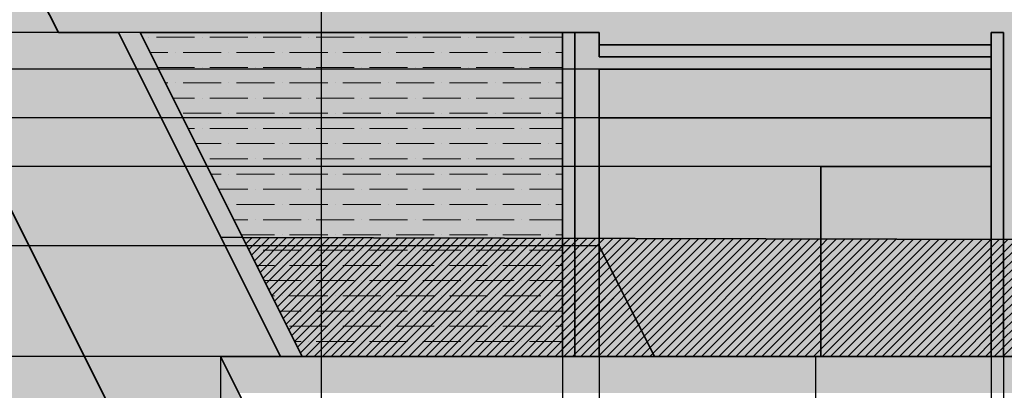
# Model space of a CAD drawing. Units: millimetres. Extents: x -504 to 6314, y 1290 to 4335.
# Tile 4 of 9: x 1774 to 3796, y 2556 to 3317. Entities that reach past the tile are written whole.
import ezdxf

# ---------------------------------------------------------------- set-up
doc = ezdxf.new("R2010")
doc.units = ezdxf.units.MM
doc.header["$MEASUREMENT"] = 0
for name, color, linetype, lineweight in [('A-ANNO-DIMS', 2, 'Continuous', 18), ('A-ELEV', 7, 'Continuous', 35), ('A-ELEV-PATT', 8, 'Continuous', 13)]:
    doc.layers.add(name, color=color, linetype=linetype, lineweight=lineweight)
doc.styles.get("Standard").update_dxf_attribs({"font": 'arial.ttf'})
doc.dimstyles.get("Standard").update_dxf_attribs({"dimtxt": 150, "dimasz": 100, "dimexe": 0.18, "dimexo": 0.0625, "dimgap": 0.09, "dimtad": 0, "dimtih": 1, "dimtoh": 1, "dimdec": 0, "dimzin": 0, "dimdsep": 46, "dimtxsty": 'Standard', "dimcen": 0.09, "dimadec": 0, "dimazin": 0, "dimtfac": 1, "dimtdec": 0, "dimtofl": 0, "dimtmove": 0, "dimatfit": 3, "dimfxl": 1, "dimtolj": 1, "dimtzin": 0, "dimarcsym": 0})
pattern_1 = [(50, (0, 0), (71.726, -6.2752), [7.5, -82.5]), (355, (0, 0), (-13.8751, 75.2192), [6, -66]), (100.4514, (5.98, -0.52), (57.8509, 68.944), [6.374, -70.1142]), (46.1842, (0, 20), (106.7241, -16.5519), [11.25, -123.75]), (96.6356, (8.89, 18.62), (93.4662, 97.4119), [9.561, -105.1714]), (351.1842, (0, 20), (93.4662, 97.4119), [9, -99]), (21, (10, 15), (59.6907, -40.2619), [7.5, -82.5]), (326, (10, 15), (24.3315, 72.515), [6, -66]), (71.4514, (14.974, 11.645), (84.0222, 32.2531), [6.374, -70.1142]), (37.5, (0, 0), (1.21599, 33.28939), [0, -65.2, 0, -67, 0, -66.25]), (7.5, (0, 0), (26.30695, 39.44117), [0, -38.2, 0, -63.7, 0, -25.25]), (327.5, (-22.3, 0), (53.38224, -2.25549), [0, -25, 0, -78, 0, -103.5]), (317.5, (-32.3, 0), (58.3186, 10.0105), [0, -32.5, 0, -51.8, 0, -73.5])]

# ---------------------------------------------------------------- blocks, each defined once
blk = doc.blocks.new('*D5')
at = {"layer": 'A-ANNO-DIMS', "color": 0, "lineweight": -2, "transparency": 16777216}
for p, q in [((4260.1, 2625.8), (5589, 2625.8)), ((5588.8, 2525.8), (5588.8, 2215.7)), ((5588.8, 1752.1), (5588.8, 2062.2)), ((72.9, 1652.1), (5589, 1652.1))]:
    blk.add_line(p, q, dxfattribs=at)
at = {"layer": 'A-ANNO-DIMS', "color": 0, "transparency": 16777216}
for points in [[(5572.1, 2525.8), (5605.5, 2525.8), (5588.8, 2625.8)], [(5572.1, 1752.1), (5605.5, 1752.1), (5588.8, 1652.1)]]:
    blk.add_solid(points, dxfattribs=at)
at = {"layer": 'Defpoints', "color": 0, "transparency": 16777216}
for p in [(4260, 2625.8), (5588.8, 2625.8), (72.8, 1652.1)]:
    blk.add_point(p, dxfattribs=at)
at = {"layer": 'A-ANNO-DIMS', "color": 0, "transparency": 16777216, "insert": (5588.8, 2138.9), "char_height": 150, "attachment_point": 5}
blk.add_mtext('\\A1;973.6', dxfattribs=at)
blk = doc.blocks.new('*D6')
at = {"layer": 'A-ANNO-DIMS', "color": 0, "lineweight": -2, "transparency": 16777216}
for p, q in [((72.8, 1652.2), (72.8, 4237)), ((172.8, 4236.8), (920.4, 4236.8)), ((2293.5, 4236.8), (1545.9, 4236.8)), ((2393.5, 1652.2), (2393.5, 4237))]:
    blk.add_line(p, q, dxfattribs=at)
at = {"layer": 'A-ANNO-DIMS', "color": 0, "transparency": 16777216}
for points in [[(172.8, 4253.4), (172.8, 4220.1), (72.8, 4236.8)], [(2293.5, 4253.4), (2293.5, 4220.1), (2393.5, 4236.8)]]:
    blk.add_solid(points, dxfattribs=at)
at = {"layer": 'Defpoints', "color": 0, "transparency": 16777216}
for p in [(2393.5, 4236.8), (72.8, 1652.1), (2393.5, 1652.1)]:
    blk.add_point(p, dxfattribs=at)
at = {"layer": 'A-ANNO-DIMS', "color": 0, "transparency": 16777216, "insert": (1233.2, 4236.8), "char_height": 150, "attachment_point": 5}
blk.add_mtext('\\A1;2320.7', dxfattribs=at)
blk = doc.blocks.new('*D28')
at = {"layer": 'A-ANNO-DIMS', "color": 0, "lineweight": -2, "transparency": 16777216}
for p, q in [((-191.2, 3540.7), (-191.2, 3640.7)), ((-191.2, 3640.7), (-91.2, 3640.7)), ((4308.5, 3440.7), (-191.3, 3440.7)), ((4304.4, 3340.7), (-191.3, 3340.7)), ((-191.2, 3240.7), (-191.2, 3140.7))]:
    blk.add_line(p, q, dxfattribs=at)
at = {"layer": 'A-ANNO-DIMS', "color": 0, "transparency": 16777216}
for points in [[(-207.8, 3540.7), (-174.5, 3540.7), (-191.2, 3440.7)], [(-207.8, 3240.7), (-174.5, 3240.7), (-191.2, 3340.7)]]:
    blk.add_solid(points, dxfattribs=at)
at = {"layer": 'Defpoints', "color": 0, "transparency": 16777216}
for p in [(-191.2, 3440.7), (4308.6, 3440.7), (4304.5, 3340.7)]:
    blk.add_point(p, dxfattribs=at)
at = {"layer": 'A-ANNO-DIMS', "color": 0, "transparency": 16777216, "insert": (67.3, 3640.7), "char_height": 150, "attachment_point": 5}
blk.add_mtext('\\A1;100', dxfattribs=at)
blk = doc.blocks.new('*D31')
at = {"layer": 'A-ANNO-DIMS', "color": 0, "lineweight": -2, "transparency": 16777216}
for p, q in [((-191.2, 2852.5), (-191.2, 2952.5)), ((-191.2, 2952.5), (-91.2, 2952.5)), ((2963.6, 2852.5), (-191.3, 2852.5)), ((-191.2, 2725.8), (-191.2, 2752.5)), ((2963.6, 2625.8), (-191.3, 2625.8))]:
    blk.add_line(p, q, dxfattribs=at)
at = {"layer": 'A-ANNO-DIMS', "color": 0, "transparency": 16777216}
for points in [[(-207.8, 2752.5), (-174.5, 2752.5), (-191.2, 2852.5)], [(-207.8, 2725.8), (-174.5, 2725.8), (-191.2, 2625.8)]]:
    blk.add_solid(points, dxfattribs=at)
at = {"layer": 'Defpoints', "color": 0, "transparency": 16777216}
for p in [(-191.2, 2852.5), (2963.6, 2852.5), (2963.6, 2625.8)]:
    blk.add_point(p, dxfattribs=at)
at = {"layer": 'A-ANNO-DIMS', "color": 0, "transparency": 16777216, "insert": (163.3, 2952.5), "char_height": 150, "attachment_point": 5}
blk.add_mtext('\\A1;226.7', dxfattribs=at)
blk = doc.blocks.new('*D32')
at = {"layer": 'A-ANNO-DIMS', "color": 0, "lineweight": -2, "transparency": 16777216}
for p, q in [((-191.2, 3115.7), (-191.2, 3215.7)), ((-191.2, 3215.7), (-91.2, 3215.7)), ((2963.6, 3115.7), (-191.3, 3115.7)), ((-191.2, 2952.5), (-191.2, 3015.7)), ((2963.6, 2852.5), (-191.3, 2852.5))]:
    blk.add_line(p, q, dxfattribs=at)
at = {"layer": 'A-ANNO-DIMS', "color": 0, "transparency": 16777216}
for points in [[(-207.8, 3015.7), (-174.5, 3015.7), (-191.2, 3115.7)], [(-207.8, 2952.5), (-174.5, 2952.5), (-191.2, 2852.5)]]:
    blk.add_solid(points, dxfattribs=at)
at = {"layer": 'Defpoints', "color": 0, "transparency": 16777216}
for p in [(-191.2, 3115.7), (2963.6, 3115.7), (2963.6, 2852.5)]:
    blk.add_point(p, dxfattribs=at)
at = {"layer": 'A-ANNO-DIMS', "color": 0, "transparency": 16777216, "insert": (162.5, 3215.7), "char_height": 150, "attachment_point": 5}
blk.add_mtext('\\A1;263.2', dxfattribs=at)
blk = doc.blocks.new('*D33')
at = {"layer": 'A-ANNO-DIMS', "color": 0, "lineweight": -2, "transparency": 16777216}
for p, q in [((-191.2, 3315.7), (-191.2, 3415.7)), ((-191.2, 3415.7), (-91.2, 3415.7)), ((2963.6, 3215.7), (-191.3, 3215.7)), ((2963.6, 3115.7), (-191.3, 3115.7)), ((-191.2, 3015.7), (-191.2, 2915.7))]:
    blk.add_line(p, q, dxfattribs=at)
at = {"layer": 'A-ANNO-DIMS', "color": 0, "transparency": 16777216}
for points in [[(-207.8, 3315.7), (-174.5, 3315.7), (-191.2, 3215.7)], [(-207.8, 3015.7), (-174.5, 3015.7), (-191.2, 3115.7)]]:
    blk.add_solid(points, dxfattribs=at)
at = {"layer": 'Defpoints', "color": 0, "transparency": 16777216}
for p in [(-191.2, 3215.7), (2963.6, 3215.7), (2963.6, 3115.7)]:
    blk.add_point(p, dxfattribs=at)
at = {"layer": 'A-ANNO-DIMS', "color": 0, "transparency": 16777216, "insert": (67.3, 3415.7), "char_height": 150, "attachment_point": 5}
blk.add_mtext('\\A1;100', dxfattribs=at)
blk = doc.blocks.new('*D34')
at = {"layer": 'A-ANNO-DIMS', "color": 0, "lineweight": -2, "transparency": 16777216}
for p, q in [((-191.2, 3390.7), (-191.2, 3490.7)), ((-191.2, 3490.7), (-91.2, 3490.7)), ((2963.6, 3290.7), (-191.3, 3290.7)), ((2963.6, 3215.7), (-191.3, 3215.7)), ((-191.2, 3115.7), (-191.2, 3015.7))]:
    blk.add_line(p, q, dxfattribs=at)
at = {"layer": 'A-ANNO-DIMS', "color": 0, "transparency": 16777216}
for points in [[(-207.8, 3390.7), (-174.5, 3390.7), (-191.2, 3290.7)], [(-207.8, 3115.7), (-174.5, 3115.7), (-191.2, 3215.7)]]:
    blk.add_solid(points, dxfattribs=at)
at = {"layer": 'Defpoints', "color": 0, "transparency": 16777216}
for p in [(-191.2, 3290.7), (2963.6, 3290.7), (2963.6, 3215.7)]:
    blk.add_point(p, dxfattribs=at)
at = {"layer": 'A-ANNO-DIMS', "color": 0, "transparency": 16777216, "insert": (16.3, 3490.7), "char_height": 150, "attachment_point": 5}
blk.add_mtext('\\A1;75', dxfattribs=at)
blk = doc.blocks.new('*D35')
at = {"layer": 'A-ANNO-DIMS', "color": 0, "lineweight": -2, "transparency": 16777216}
for p, q in [((3418.6, 3015.7), (-191.3, 3015.7)), ((-191.2, 2915.7), (-191.2, 2897.4)), ((-191.2, 2725.8), (-191.2, 2744)), ((3407.7, 2625.8), (-191.3, 2625.8))]:
    blk.add_line(p, q, dxfattribs=at)
at = {"layer": 'A-ANNO-DIMS', "color": 0, "transparency": 16777216}
for points in [[(-207.8, 2915.7), (-174.5, 2915.7), (-191.2, 3015.7)], [(-207.8, 2725.8), (-174.5, 2725.8), (-191.2, 2625.8)]]:
    blk.add_solid(points, dxfattribs=at)
at = {"layer": 'Defpoints', "color": 0, "transparency": 16777216}
for p in [(-191.2, 3015.7), (3418.6, 3015.7), (3407.8, 2625.8)]:
    blk.add_point(p, dxfattribs=at)
at = {"layer": 'A-ANNO-DIMS', "color": 0, "transparency": 16777216, "insert": (-191.2, 2820.7), "char_height": 150, "attachment_point": 5}
blk.add_mtext('\\A1;389.9', dxfattribs=at)
blk = doc.blocks.new('*D36')
at = {"layer": 'A-ANNO-DIMS', "color": 0, "lineweight": -2, "transparency": 16777216}
for p, q in [((2186.2, 2625.7), (2186.2, 1387.9)), ((2888.6, 2625.7), (2888.6, 1387.9)), ((2086.2, 1388.1), (1986.2, 1388.1)), ((2988.6, 1388.1), (3088.6, 1388.1))]:
    blk.add_line(p, q, dxfattribs=at)
at = {"layer": 'A-ANNO-DIMS', "color": 0, "transparency": 16777216}
for points in [[(2086.2, 1404.8), (2086.2, 1371.5), (2186.2, 1388.1)], [(2988.6, 1404.8), (2988.6, 1371.5), (2888.6, 1388.1)]]:
    blk.add_solid(points, dxfattribs=at)
at = {"layer": 'Defpoints', "color": 0, "transparency": 16777216}
for p in [(2186.2, 2625.8), (2888.6, 2625.8), (2888.6, 1388.1)]:
    blk.add_point(p, dxfattribs=at)
at = {"layer": 'A-ANNO-DIMS', "color": 0, "transparency": 16777216, "insert": (2537.4, 1388.1), "char_height": 150, "attachment_point": 5}
blk.add_mtext('\\A1;702.5', dxfattribs=at)
blk = doc.blocks.new('*D37')
at = {"layer": 'A-ANNO-DIMS', "color": 0, "lineweight": -2, "transparency": 16777216}
for p, q in [((2888.6, 2625.7), (2888.6, 1387.9)), ((2963.6, 2625.7), (2963.6, 1387.9)), ((2788.6, 1388.1), (2688.6, 1388.1)), ((3063.6, 1388.1), (3163.6, 1388.1))]:
    blk.add_line(p, q, dxfattribs=at)
at = {"layer": 'A-ANNO-DIMS', "color": 0, "transparency": 16777216}
for points in [[(2788.6, 1404.8), (2788.6, 1371.5), (2888.6, 1388.1)], [(3063.6, 1404.8), (3063.6, 1371.5), (2963.6, 1388.1)]]:
    blk.add_solid(points, dxfattribs=at)
at = {"layer": 'Defpoints', "color": 0, "transparency": 16777216}
for p in [(2888.6, 2625.8), (2963.6, 2625.8), (2963.6, 1388.1)]:
    blk.add_point(p, dxfattribs=at)
at = {"layer": 'A-ANNO-DIMS', "color": 0, "transparency": 16777216, "insert": (3271.1, 1388.1), "char_height": 150, "attachment_point": 5}
blk.add_mtext('\\A1;75', dxfattribs=at)
blk = doc.blocks.new('*D38')
at = {"layer": 'A-ANNO-DIMS', "color": 0, "lineweight": -2, "transparency": 16777216}
for p, q in [((2963.6, 2625.7), (2963.6, 1387.9)), ((3407.8, 2625.7), (3407.8, 1387.9)), ((3063.6, 1388.1), (3307.8, 1388.1)), ((3407.8, 1388.1), (3507.8, 1388.1))]:
    blk.add_line(p, q, dxfattribs=at)
at = {"layer": 'A-ANNO-DIMS', "color": 0, "transparency": 16777216}
for points in [[(3063.6, 1404.8), (3063.6, 1371.5), (2963.6, 1388.1)], [(3307.8, 1404.8), (3307.8, 1371.5), (3407.8, 1388.1)]]:
    blk.add_solid(points, dxfattribs=at)
at = {"layer": 'Defpoints', "color": 0, "transparency": 16777216}
for p in [(2963.6, 2625.8), (3407.8, 2625.8), (3407.8, 1388.1)]:
    blk.add_point(p, dxfattribs=at)
at = {"layer": 'A-ANNO-DIMS', "color": 0, "transparency": 16777216, "insert": (3763.2, 1388.1), "char_height": 150, "attachment_point": 5}
blk.add_mtext('\\A1;444.2', dxfattribs=at)
blk = doc.blocks.new('*D39')
at = {"layer": 'A-ANNO-DIMS', "color": 0, "lineweight": -2, "transparency": 16777216}
for p, q in [((3407.8, 2625.7), (3407.8, 1387.9)), ((3768.6, 2625.7), (3768.6, 1387.9)), ((3507.8, 1388.1), (3668.6, 1388.1)), ((3768.6, 1388.1), (3868.6, 1388.1))]:
    blk.add_line(p, q, dxfattribs=at)
at = {"layer": 'A-ANNO-DIMS', "color": 0, "transparency": 16777216}
for points in [[(3507.8, 1404.8), (3507.8, 1371.5), (3407.8, 1388.1)], [(3668.6, 1404.8), (3668.6, 1371.5), (3768.6, 1388.1)]]:
    blk.add_solid(points, dxfattribs=at)
at = {"layer": 'Defpoints', "color": 0, "transparency": 16777216}
for p in [(3407.8, 2625.8), (3768.6, 2625.8), (3768.6, 1388.1)]:
    blk.add_point(p, dxfattribs=at)
at = {"layer": 'A-ANNO-DIMS', "color": 0, "transparency": 16777216, "insert": (4179.7, 1388.1), "char_height": 150, "attachment_point": 5}
blk.add_mtext('\\A1;360.84', dxfattribs=at)
blk = doc.blocks.new('*D40')
at = {"layer": 'A-ANNO-DIMS', "color": 0, "lineweight": -2, "transparency": 16777216}
for p, q in [((3768.6, 2625.7), (3768.6, 1387.9)), ((3793.6, 2625.7), (3793.6, 1387.9)), ((3668.6, 1388.1), (3568.6, 1388.1)), ((3893.6, 1388.1), (3993.6, 1388.1))]:
    blk.add_line(p, q, dxfattribs=at)
at = {"layer": 'A-ANNO-DIMS', "color": 0, "transparency": 16777216}
for points in [[(3668.6, 1404.8), (3668.6, 1371.5), (3768.6, 1388.1)], [(3893.6, 1404.8), (3893.6, 1371.5), (3793.6, 1388.1)]]:
    blk.add_solid(points, dxfattribs=at)
at = {"layer": 'Defpoints', "color": 0, "transparency": 16777216}
for p in [(3768.6, 2625.8), (3793.6, 2625.8), (3793.6, 1388.1)]:
    blk.add_point(p, dxfattribs=at)
at = {"layer": 'A-ANNO-DIMS', "color": 0, "transparency": 16777216, "insert": (4103, 1388.1), "char_height": 150, "attachment_point": 5}
blk.add_mtext('\\A1;25', dxfattribs=at)
blk = doc.blocks.new('*D41')
at = {"layer": 'A-ANNO-DIMS', "color": 0, "lineweight": -2, "transparency": 16777216}
for p, q in [((3793.6, 2625.7), (3793.6, 1387.9)), ((3818.6, 2625.7), (3818.6, 1387.9)), ((3693.6, 1388.1), (3593.6, 1388.1)), ((3918.6, 1388.1), (4018.6, 1388.1))]:
    blk.add_line(p, q, dxfattribs=at)
at = {"layer": 'A-ANNO-DIMS', "color": 0, "transparency": 16777216}
for points in [[(3693.6, 1404.8), (3693.6, 1371.5), (3793.6, 1388.1)], [(3918.6, 1404.8), (3918.6, 1371.5), (3818.6, 1388.1)]]:
    blk.add_solid(points, dxfattribs=at)
at = {"layer": 'Defpoints', "color": 0, "transparency": 16777216}
for p in [(3793.6, 2625.8), (3818.6, 2625.8), (3818.6, 1388.1)]:
    blk.add_point(p, dxfattribs=at)
at = {"layer": 'A-ANNO-DIMS', "color": 0, "transparency": 16777216, "insert": (4128, 1388.1), "char_height": 150, "attachment_point": 5}
blk.add_mtext('\\A1;25', dxfattribs=at)
blk = doc.blocks.new('*D42')
at = {"layer": 'A-ANNO-DIMS', "color": 0, "lineweight": -2, "transparency": 16777216}
for p, q in [((3818.6, 2625.7), (3818.6, 1387.9)), ((4198.6, 2625.7), (4198.6, 1387.9)), ((3718.6, 1388.1), (3618.6, 1388.1)), ((4298.6, 1388.1), (4398.6, 1388.1))]:
    blk.add_line(p, q, dxfattribs=at)
at = {"layer": 'A-ANNO-DIMS', "color": 0, "transparency": 16777216}
for points in [[(3718.6, 1404.8), (3718.6, 1371.5), (3818.6, 1388.1)], [(4298.6, 1404.8), (4298.6, 1371.5), (4198.6, 1388.1)]]:
    blk.add_solid(points, dxfattribs=at)
at = {"layer": 'Defpoints', "color": 0, "transparency": 16777216}
for p in [(3818.6, 2625.8), (4198.6, 2625.8), (4198.6, 1388.1)]:
    blk.add_point(p, dxfattribs=at)
at = {"layer": 'A-ANNO-DIMS', "color": 0, "transparency": 16777216, "insert": (4008.6, 1388.1), "char_height": 150, "attachment_point": 5}
blk.add_mtext('\\A1;380', dxfattribs=at)
blk = doc.blocks.new('*D66')
at = {"layer": 'A-ANNO-DIMS', "color": 0, "lineweight": -2, "transparency": 16777216}
for p, q in [((3753.7, 4236.8), (3653.7, 4236.8)), ((3853.7, 1932.9), (3853.7, 4237)), ((3992.1, 1982.9), (3992.1, 4237)), ((4092.1, 4236.8), (4192.1, 4236.8))]:
    blk.add_line(p, q, dxfattribs=at)
at = {"layer": 'A-ANNO-DIMS', "color": 0, "transparency": 16777216}
for points in [[(3753.7, 4253.4), (3753.7, 4220.1), (3853.7, 4236.8)], [(4092.1, 4253.4), (4092.1, 4220.1), (3992.1, 4236.8)]]:
    blk.add_solid(points, dxfattribs=at)
at = {"layer": 'Defpoints', "color": 0, "transparency": 16777216}
for p in [(3992.1, 4236.8), (3992.1, 1982.8), (3853.7, 1932.8)]:
    blk.add_point(p, dxfattribs=at)
at = {"layer": 'A-ANNO-DIMS', "color": 0, "transparency": 16777216, "insert": (4496.6, 4236.8), "char_height": 150, "attachment_point": 5}
blk.add_mtext('\\A1;138.38', dxfattribs=at)
blk = doc.blocks.new('*D69')
at = {"layer": 'A-ANNO-DIMS', "color": 0, "lineweight": -2, "transparency": 16777216}
for p, q in [((-191.2, 2625.8), (-191.2, 2725.8)), ((-191.2, 2725.8), (-91.2, 2725.8)), ((3076.9, 2525.8), (-191.3, 2525.8)), ((3076.9, 2475.8), (-191.3, 2475.8)), ((-191.2, 2375.8), (-191.2, 2275.8))]:
    blk.add_line(p, q, dxfattribs=at)
at = {"layer": 'A-ANNO-DIMS', "color": 0, "transparency": 16777216}
for points in [[(-207.8, 2625.8), (-174.5, 2625.8), (-191.2, 2525.8)], [(-207.8, 2375.8), (-174.5, 2375.8), (-191.2, 2475.8)]]:
    blk.add_solid(points, dxfattribs=at)
at = {"layer": 'Defpoints', "color": 0, "transparency": 16777216}
for p in [(-191.2, 2525.8), (3077, 2525.8), (3077, 2475.8)]:
    blk.add_point(p, dxfattribs=at)
at = {"layer": 'A-ANNO-DIMS', "color": 0, "transparency": 16777216, "insert": (16.1, 2725.8), "char_height": 150, "attachment_point": 5}
blk.add_mtext('\\A1;50', dxfattribs=at)
blk = doc.blocks.new('*D74')
at = {"layer": 'A-ANNO-DIMS', "color": 0, "lineweight": -2, "transparency": 16777216}
for p, q in [((-191.2, 2475.8), (-191.2, 2575.8)), ((-191.2, 2575.8), (-91.2, 2575.8)), ((3447.7, 2475.8), (-191.3, 2475.8)), ((-191.2, 2334.8), (-191.2, 2375.8)), ((3447.7, 2234.8), (-191.3, 2234.8))]:
    blk.add_line(p, q, dxfattribs=at)
at = {"layer": 'A-ANNO-DIMS', "color": 0, "transparency": 16777216}
for points in [[(-207.8, 2375.8), (-174.5, 2375.8), (-191.2, 2475.8)], [(-207.8, 2334.8), (-174.5, 2334.8), (-191.2, 2234.8)]]:
    blk.add_solid(points, dxfattribs=at)
at = {"layer": 'Defpoints', "color": 0, "transparency": 16777216}
for p in [(-191.2, 2475.8), (3447.8, 2475.8), (3447.8, 2234.8)]:
    blk.add_point(p, dxfattribs=at)
at = {"layer": 'A-ANNO-DIMS', "color": 0, "transparency": 16777216, "insert": (61.4, 2575.8), "char_height": 150, "attachment_point": 5}
blk.add_mtext('\\A1;241', dxfattribs=at)

msp = doc.modelspace()

# ---------------------------------------------------------------- hatches: boundary and pattern name
at = {"layer": 'A-ELEV-PATT'}
for points in [[(3324.48, 3780.626), (1233.163, 3972.781), (72.835, 1652.125), (2393.491, 1652.125), (2355.991, 1727.125), (138.286, 1727.125), (1247.138, 3944.83), (2393.491, 1652.125), (2840.705, 1652.125), (2403.888, 2525.758), (2236.182, 2525.758), (2186.182, 2625.758), (2309.166, 2625.758), (1976.702, 3290.687), (1853.718, 3290.687), (1778.718, 3440.687), (3407.797, 3440.687)], [(3768.634, 3215.687), (3407.797, 3215.687), (2963.634, 3215.687), (2963.634, 3115.687), (3768.634, 3115.687)], [(3418.634, 3015.687), (3768.634, 3015.687), (3768.634, 3115.687), (2963.634, 3115.687), (2963.634, 2852.466), (3076.987, 2625.758), (3407.797, 2625.758), (3418.634, 2625.758)], [(5324.792, 2261.16), (5324.792, 2338.836), (4260.021, 2625.758), (3929.687, 2625.758), (3407.797, 2625.758), (2186.182, 2625.758), (2223.682, 2550.758), (3407.797, 2550.758), (3929.687, 2550.758), (4250.093, 2550.758)]]:
    msp.add_hatch(color=256, dxfattribs=at).paths.add_polyline_path(points)
h = msp.add_hatch(dxfattribs=at)
h.set_pattern_fill('ANSI36', color=256, scale=200, angle=135, style=0)
h.paths.add_polyline_path([(3324.48, 3780.626), (1233.163, 3972.781), (72.835, 1652.125), (2393.491, 1652.125), (2355.991, 1727.125), (138.286, 1727.125), (1247.138, 3944.83), (2393.491, 1652.125), (2840.705, 1652.125), (2403.888, 2525.758), (2236.182, 2525.758), (2186.182, 2625.758), (2309.166, 2625.758), (1976.702, 3290.687), (1853.718, 3290.687), (1778.718, 3440.687), (3407.797, 3440.687)])
h = msp.add_hatch(dxfattribs=at)
h.set_pattern_fill('AR-CONC', color=256, scale=10, style=0)
h.set_pattern_definition(pattern_1)
h.paths.add_polyline_path([(4308.57, 3440.687), (3929.687, 3440.687), (3407.797, 3440.687), (1778.718, 3440.687), (1828.718, 3340.687), (3407.797, 3340.687), (3929.687, 3340.687), (4304.463, 3340.687), (5081.168, 3138.941), (5082.876, 3139.564), (5082.876, 3239.564)])
h.paths.add_polyline_path([(4260.021, 2625.758), (3929.687, 2625.758), (3407.797, 2625.758), (2186.182, 2625.758), (2223.682, 2550.758), (3407.797, 2550.758), (3929.687, 2550.758), (4250.093, 2550.758), (5324.792, 2261.16), (5324.792, 2338.836)])
h = msp.add_hatch(color=256, dxfattribs=at)
h.paths.add_polyline_path([(4304.463, 3340.687), (3929.687, 3340.687), (3407.797, 3340.687), (1828.718, 3340.687), (1853.718, 3290.687), (1976.702, 3290.687), (2309.166, 2625.758), (2353.888, 2625.758), (2021.423, 3290.687), (2963.634, 3290.687), (2963.634, 3265.687), (3407.797, 3265.687), (3768.634, 3265.687), (3768.634, 3290.687), (3793.634, 3290.687), (3793.634, 2625.758), (3818.634, 2625.758), (3818.634, 3290.687), (3929.687, 3290.687), (4198.634, 3290.687), (4473.634, 3219.257), (4473.634, 2568.197), (4498.634, 2561.46), (4498.634, 3167.307), (4673.634, 3167.307), (4923.634, 3102.371), (4923.634, 3081.487), (5081.168, 3138.941)])
h.paths.add_polyline_path([(3768.634, 3240.687), (3407.797, 3240.687), (2963.634, 3240.687), (2963.634, 3290.687), (2913.634, 3290.687), (2913.634, 2625.758), (2963.634, 2625.758), (2963.634, 3215.687), (3407.797, 3215.687), (3768.634, 3215.687)], flags=17)
h = msp.add_hatch(color=256, dxfattribs=at)
h.paths.add_polyline_path([(2888.634, 3290.687), (2021.423, 3290.687), (2353.888, 2625.758), (2888.634, 2625.758)])
h.paths.add_polyline_path([(4198.634, 3290.687), (3929.687, 3290.687), (3818.634, 3290.687), (3818.634, 2625.758), (3929.687, 2625.758), (4198.634, 2625.758)])
h.paths.add_polyline_path([(4473.634, 3219.257), (4198.634, 3290.687), (4198.634, 2625.758), (4260.021, 2625.758), (4473.634, 2568.197)])
h.paths.add_polyline_path([(4673.634, 3167.307), (4498.634, 3167.307), (4498.634, 2561.46), (4673.634, 2514.303)])
h.paths.add_polyline_path([(4923.634, 3102.371), (4673.634, 3167.307), (4673.634, 2514.303), (4923.634, 2446.935)])
h = msp.add_hatch(dxfattribs=at)
h.set_pattern_fill('ANSI36', color=256, scale=250, angle=135, style=0)
h.paths.add_polyline_path([(2888.634, 3290.687), (2021.423, 3290.687), (2231.996, 2869.543), (2888.634, 2868.048)])
h.paths.add_polyline_path([(4198.634, 3290.687), (3929.687, 3290.687), (3818.634, 3290.687), (3818.634, 2865.931), (4198.634, 2865.066)])
h.paths.add_polyline_path([(4473.634, 3219.257), (4198.634, 3290.687), (4198.634, 2865.066), (4473.634, 2864.44)])
h.paths.add_polyline_path([(4923.634, 3102.371), (4673.634, 3167.307), (4673.634, 2814.647), (4923.634, 2747.28)])
h.paths.add_polyline_path([(4673.634, 3167.307), (4498.634, 3167.307), (4498.634, 2861.804), (4673.634, 2814.647)])
h.paths.add_polyline_path([(4673.634, 2814.647), (4498.634, 2861.804), (4498.634, 2561.46), (4673.634, 2514.303)])
h.paths.add_polyline_path([(4923.634, 2747.28), (4673.634, 2814.647), (4673.634, 2514.303), (4923.634, 2446.935)])
h.paths.add_polyline_path([(4473.634, 2864.44), (4198.634, 2865.066), (4198.634, 2625.758), (4260.021, 2625.758), (4473.634, 2568.197)])
h.paths.add_polyline_path([(4198.634, 2865.066), (3818.634, 2865.931), (3818.634, 2625.758), (3929.687, 2625.758), (4198.634, 2625.758)])
h.paths.add_polyline_path([(2888.634, 2868.048), (2231.996, 2869.543), (2353.888, 2625.758), (2888.634, 2625.758)])
h = msp.add_hatch(color=256, dxfattribs=at)
h.paths.add_polyline_path([(2913.634, 3290.687), (2888.634, 3290.687), (2888.634, 2868.048), (2913.634, 2867.991)])
h.paths.add_polyline_path([(3793.634, 3290.687), (3768.634, 3290.687), (3768.634, 2866.045), (3793.634, 2865.988)])
h.paths.add_polyline_path([(3793.634, 2865.988), (3768.634, 2866.045), (3768.634, 2625.758), (3793.634, 2625.758)])
h.paths.add_polyline_path([(2913.634, 2867.991), (2888.634, 2868.048), (2888.634, 2625.758), (2913.634, 2625.758)])
h = msp.add_hatch(color=256, dxfattribs=at)
h.paths.add_polyline_path([(3768.634, 3265.687), (3407.797, 3265.687), (2963.634, 3265.687), (2963.634, 3240.687), (3407.797, 3240.687), (3768.634, 3240.687)])
h.paths.add_polyline_path([(2963.634, 2852.466), (2963.634, 2625.758), (3076.987, 2625.758)])
h.paths.add_polyline_path([(3768.634, 3015.687), (3418.634, 3015.687), (3418.634, 2625.758), (3768.634, 2625.758)])
h = msp.add_hatch(color=256, dxfattribs=at)
h.set_gradient(color1=(99, 100, 102), color2=(254, 204, 102), name='CYLINDER')
h.paths.add_polyline_path([(1688.991, 3061.125), (1688.991, 2485.278), (1977.097, 2484.912)])
h.paths.add_polyline_path([(997.991, 3111.125), (685.705, 2486.552), (997.991, 2486.156)])
h = msp.add_hatch(color=256, dxfattribs=at)
h.set_gradient(color1=(147, 149, 152), color2=(254, 204, 102), tint=1, name='HEMISPHERICAL')
h.paths.add_polyline_path([(1688.991, 3061.125), (1688.991, 2485.278), (1977.097, 2484.912)])
h = msp.add_hatch(dxfattribs=at)
h.set_pattern_fill('ANSI31', color=256, scale=100, style=0)
h.paths.add_polyline_path([(2888.634, 2868.048), (2231.996, 2869.543), (2353.888, 2625.758), (2888.634, 2625.758)])
h.paths.add_polyline_path([(2913.634, 2867.991), (2888.634, 2868.048), (2888.634, 2625.758), (2913.634, 2625.758)])
h.paths.add_polyline_path([(2963.634, 2867.877), (2913.634, 2867.991), (2913.634, 2625.758), (2963.634, 2625.758)])
h.paths.add_polyline_path([(2963.634, 2852.466), (2963.634, 2625.758), (3076.987, 2625.758)], flags=17)
h.paths.add_polyline_path([(3418.634, 2866.842), (2963.634, 2867.877), (2963.634, 2852.466), (3076.987, 2625.758), (3407.797, 2625.758), (3418.634, 2625.758)])
h.paths.add_polyline_path([(3793.634, 2865.988), (3768.634, 2866.045), (3768.634, 2625.758), (3793.634, 2625.758)])
h.paths.add_polyline_path([(3818.634, 2865.931), (3793.634, 2865.988), (3793.634, 2625.758), (3818.634, 2625.758)])
h.paths.add_polyline_path([(4198.634, 2865.066), (3818.634, 2865.931), (3818.634, 2625.758), (3929.687, 2625.758), (4198.634, 2625.758)])
h.paths.add_polyline_path([(4473.634, 2864.44), (4198.634, 2865.066), (4198.634, 2625.758), (4260.021, 2625.758), (4473.634, 2568.197)])
h.paths.add_polyline_path([(4673.634, 2814.647), (4498.634, 2861.804), (4498.634, 2561.46), (4673.634, 2514.303)])
h.paths.add_polyline_path([(4923.634, 2747.28), (4673.634, 2814.647), (4673.634, 2514.303), (4923.634, 2446.935)])
h.paths.add_polyline_path([(5297.748, 2636.111), (4923.634, 2736.923), (4923.634, 2512.3), (5028.262, 2557.166)])
h.paths.add_polyline_path([(5028.284, 2546.295), (4923.634, 2501.42), (4923.634, 2446.935), (5028.548, 2418.664)])
h.paths.add_polyline_path([(5316.163, 2631.085), (5031.65, 2547.739), (5028.284, 2546.295), (5028.548, 2418.664), (5316.163, 2341.161)])
h = msp.add_hatch(dxfattribs=at)
h.set_pattern_fill('ANSI31', color=256, scale=100, style=0)
h.paths.add_polyline_path([(2963.634, 2852.466), (2963.634, 2625.758), (3076.987, 2625.758)], flags=17)
h.paths.add_polyline_path([(3418.634, 2866.842), (2963.634, 2867.877), (2963.634, 2852.466), (3076.987, 2625.758), (3407.797, 2625.758), (3418.634, 2625.758)])
h.paths.add_polyline_path([(2913.634, 2867.991), (2888.634, 2868.048), (2888.634, 2625.758), (2913.634, 2625.758)])
h.paths.add_polyline_path([(2963.634, 2852.466), (2963.634, 2867.877), (2913.634, 2867.991), (2913.634, 2625.758), (2963.634, 2625.758)])
h = msp.add_hatch(dxfattribs=at)
h.set_pattern_fill('ANSI31', color=256, scale=100, style=0)
h.paths.add_polyline_path([(3768.634, 2866.045), (3418.634, 2866.842), (3418.634, 2625.758), (3768.634, 2625.758)])
h = msp.add_hatch(dxfattribs=at)
h.set_pattern_fill('ANSI31', color=256, scale=100, style=0)
h.paths.add_polyline_path([(3793.634, 2865.988), (3768.634, 2866.045), (3768.634, 2625.758), (3793.634, 2625.758)])
h.paths.add_polyline_path([(4498.634, 2861.804), (4488.98, 2864.406), (4473.634, 2864.44), (4473.634, 2568.197), (4498.634, 2561.46)])
h = msp.add_hatch(dxfattribs=at)
h.set_pattern_fill('AR-CONC', color=256, scale=10, style=0)
h.set_pattern_definition(pattern_1)
h.paths.add_polyline_path([(4260.021, 2625.758), (3929.687, 2625.758), (3407.797, 2625.758), (2186.182, 2625.758), (2223.682, 2550.758), (3407.797, 2550.758), (3929.687, 2550.758), (4250.093, 2550.758), (5324.792, 2261.16), (5324.792, 2338.836)])

# ---------------------------------------------------------------- linework, layer by layer
at = {"layer": 'A-ELEV'}
for p, q in [((1247.138, 3944.83), (2393.491, 1652.125)), ((1778.718, 3440.687), (1853.718, 3290.687)), ((1976.702, 3290.687), (1853.718, 3290.687)), ((1976.702, 3290.687), (2309.166, 2625.758)), ((2963.634, 3290.687), (2021.423, 3290.687)), ((2021.423, 3290.687), (2353.888, 2625.758)), ((2888.634, 3290.687), (2888.634, 2625.758)), ((2913.634, 3290.687), (2913.634, 2625.758)), ((2963.634, 3290.687), (2963.634, 3240.687)), ((3768.634, 3290.687), (3793.634, 3290.687)), ((3768.634, 3290.687), (3768.634, 2625.758)), ((3793.634, 3290.687), (3793.634, 2625.758)), ((2963.634, 3265.687), (3407.797, 3265.687)), ((3407.797, 3265.687), (3768.634, 3265.687)), ((2963.634, 3240.687), (3407.797, 3240.687)), ((3407.797, 3240.687), (3768.634, 3240.687)), ((2963.634, 3215.687), (3407.797, 3215.687)), ((2963.634, 3215.687), (2963.634, 2625.758)), ((3407.797, 3215.687), (3768.634, 3215.687)), ((2963.634, 3115.687), (3768.634, 3115.687)), ((3418.634, 3015.687), (3768.634, 3015.687)), ((3418.634, 3015.687), (3418.634, 2625.758)), ((2231.996, 2869.543), (2186.873, 2870.345)), ((2231.996, 2869.543), (4488.98, 2864.406)), ((2963.634, 2852.466), (3076.987, 2625.758)), ((2186.182, 2625.758), (3407.797, 2625.758)), ((2186.182, 2625.758), (2236.182, 2525.758)), ((3407.797, 2625.758), (3929.687, 2625.758))]:
    msp.add_line(p, q, dxfattribs=at)

# ---------------------------------------------------------------- dimensions: what is measured, and where the dimension line sits
at = {"layer": 'A-ANNO-DIMS'}
for base, p1, p2, override, picture, middle in [((2393.491, 4236.781), (72.835, 1652.125), (2393.491, 1652.125), {"dimdec": 1, "dimlfac": 1, "dimrnd": 0, "dimzin": 0, "dimdsep": 46, "dimlunit": 2}, '*D6', (1233.163, 4236.781)), ((3992.087, 4236.781), (3853.708, 1932.831), (3992.087, 1982.831), {"dimdec": 2, "dimlfac": 1, "dimrnd": 0, "dimzin": 0, "dimdsep": 46, "dimlunit": 2}, '*D66', (4496.628, 4236.781)), ((2888.634, 1388.125), (2186.182, 2625.758), (2888.634, 2625.758), {"dimdec": 1, "dimlfac": 1, "dimrnd": 0, "dimzin": 0, "dimdsep": 46, "dimlunit": 2}, '*D36', (2537.408, 1388.125)), ((2963.634, 1388.125), (2888.634, 2625.758), (2963.634, 2625.758), {"dimdec": 0, "dimlfac": 1, "dimrnd": 0, "dimzin": 0, "dimdsep": 46, "dimlunit": 2}, '*D37', (3271.108, 1388.125)), ((3407.797, 1388.125), (2963.634, 2625.758), (3407.797, 2625.758), {"dimdec": 1, "dimlfac": 1, "dimrnd": 0, "dimzin": 0, "dimdsep": 46, "dimlunit": 2}, '*D38', (3763.224, 1388.125)), ((3768.634, 1388.125), (3407.797, 2625.758), (3768.634, 2625.758), {"dimdec": 2, "dimlfac": 1, "dimrnd": 0, "dimzin": 0, "dimdsep": 46, "dimlunit": 2}, '*D39', (4179.723, 1388.125)), ((3793.634, 1388.125), (3768.634, 2625.758), (3793.634, 2625.758), {"dimdec": 0, "dimlfac": 1, "dimrnd": 0, "dimzin": 0, "dimdsep": 46, "dimlunit": 2}, '*D40', (4103.001, 1388.125)), ((3818.634, 1388.125), (3793.634, 2625.758), (3818.634, 2625.758), {"dimdec": 0, "dimlfac": 1, "dimrnd": 0, "dimzin": 0, "dimdsep": 46, "dimlunit": 2}, '*D41', (4128.001, 1388.125)), ((4198.634, 1388.125), (3818.634, 2625.758), (4198.634, 2625.758), {"dimdec": 0, "dimlfac": 1, "dimrnd": 0, "dimzin": 0, "dimdsep": 46, "dimlunit": 2}, '*D42', (4008.634, 1388.125))]:
    dim = msp.add_linear_dim(base=base, p1=p1, p2=p2, dimstyle='Standard', override=override, dxfattribs=at)
    dim.commit()
    dim.dimension.update_dxf_attribs({"geometry": picture, "text_midpoint": middle})
for base, p1, p2, override, picture, middle in [((-191.165, 3440.687), (4304.463, 3340.687), (4308.57, 3440.687), {"dimdec": 0, "dimlfac": 1, "dimrnd": 0, "dimzin": 0, "dimdsep": 46, "dimlunit": 2}, '*D28', (67.315, 3640.687)), ((-191.165, 3290.687), (2963.634, 3215.687), (2963.634, 3290.687), {"dimdec": 0, "dimlfac": 1, "dimrnd": 0, "dimzin": 0, "dimdsep": 46, "dimlunit": 2}, '*D34', (16.309, 3490.687)), ((-191.165, 3215.687), (2963.634, 3115.687), (2963.634, 3215.687), {"dimdec": 0, "dimlfac": 1, "dimrnd": 0, "dimzin": 0, "dimdsep": 46, "dimlunit": 2}, '*D33', (67.315, 3415.687)), ((-191.165, 3115.687), (2963.634, 2852.466), (2963.634, 3115.687), {"dimdec": 1, "dimlfac": 1, "dimrnd": 0, "dimzin": 0, "dimdsep": 46, "dimlunit": 2}, '*D32', (162.523, 3215.687)), ((-191.165, 2852.466), (2963.634, 2625.758), (2963.634, 2852.466), {"dimdec": 1, "dimlfac": 1, "dimrnd": 0, "dimzin": 0, "dimdsep": 46, "dimlunit": 2}, '*D31', (163.291, 2952.466)), ((-191.165, 3015.687), (3407.797, 2625.758), (3418.634, 3015.687), {"dimdec": 1, "dimlfac": 1, "dimrnd": 0, "dimzin": 0, "dimdsep": 46, "dimlunit": 2}, '*D35', (-191.165, 2820.723)), ((-191.165, 2525.758), (3076.987, 2475.758), (3076.987, 2525.758), {"dimdec": 0, "dimlfac": 1, "dimrnd": 0, "dimzin": 0, "dimdsep": 46, "dimlunit": 2}, '*D69', (16.104, 2725.758)), ((-191.165, 2475.758), (3447.81, 2234.758), (3447.81, 2475.758), {"dimdec": 0, "dimlfac": 1, "dimrnd": 0, "dimzin": 0, "dimdsep": 46, "dimlunit": 2}, '*D74', (61.432, 2575.758)), ((5588.792, 2625.758), (72.835, 1652.125), (4260.021, 2625.758), {"dimdec": 1, "dimlfac": 1, "dimrnd": 0, "dimzin": 0, "dimdsep": 46, "dimlunit": 2}, '*D5', (5588.792, 2138.941))]:
    dim = msp.add_linear_dim(base=base, p1=p1, p2=p2, angle=90, dimstyle='Standard', override=override, dxfattribs=at)
    dim.commit()
    dim.dimension.update_dxf_attribs({"geometry": picture, "text_midpoint": middle})

doc.saveas('drawing.dxf')
